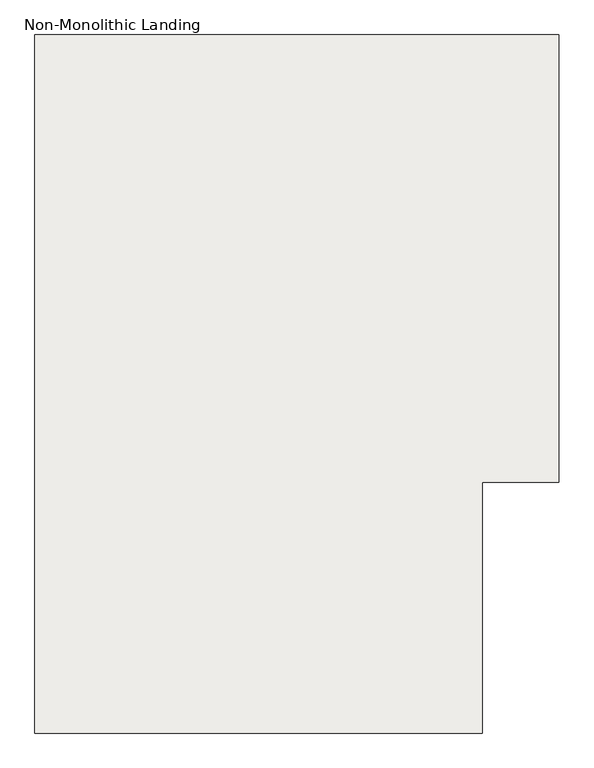
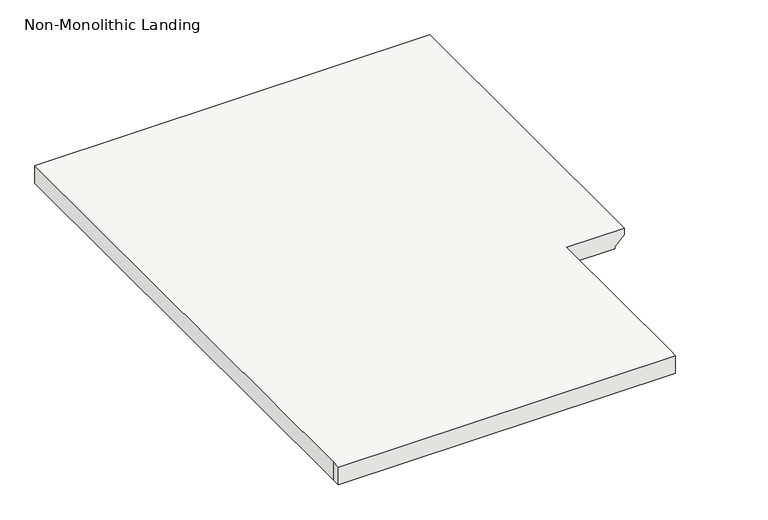
"""IFC4 building model written with IfcOpenShell, lengths in millimetres: slab geometry, Non-Monolithic Landing."""

from ifc_helpers import new_model, si_unit, origin, place, context, project, spatial, faceted_brep, source, transform, mapped, element, save


def non_monolithic_landing_30da2899(model_context):
    return source(origin(), model_context, "Body", "Brep", [
        faceted_brep([(-10197.3156858, 1045.1115003, 4180.4166667), (-10197.3156858, 1045.1115003, 4199.4666667), (-10197.3156858, 130.7115003, 4199.4666667), (-10197.3156858, 130.7115003, 4180.4166667), (-10222.7156858, 1045.1115003, 4155.0166667), (-10222.7156858, 130.7115003, 4155.0166667), (-11268.1522729, 1045.1115003, 4199.4666667), (-11268.1522729, -356.3993654, 4199.4666667), (-11268.1522729, -381.7993654, 4199.4666667), (-10353.7522729, -381.7993654, 4199.4666667), (-10353.7522729, -356.3993654, 4199.4666667), (-10353.7522729, 130.7115003, 4199.4666667), (-10222.7156858, 1045.1115003, 4148.6666667), (-10222.7156858, 130.7115003, 4148.6666667), (-10353.7522729, 130.7115003, 4148.6666667), (-10353.7522729, -356.3993654, 4148.6666667), (-10353.7522729, -381.7993654, 4148.6666667), (-11268.1522729, -381.7993654, 4148.6666667), (-11268.1522729, -356.3993654, 4148.6666667), (-11268.1522729, 1045.1115003, 4148.6666667)], [[[0, 1, 2, 3]], [[4, 0, 3, 5]], [[6, 7, 8, 9, 10, 11, 2, 1]], [[12, 13, 14, 15, 16, 17, 18, 19]], [[13, 12, 4, 5]], [[6, 1, 0, 4, 12, 19]], [[7, 6, 19, 18]], [[8, 7, 18, 17]], [[9, 8, 17, 16]], [[10, 9, 16, 15]], [[11, 10, 15, 14]], [[2, 11, 14, 13, 5, 3]]]),
    ])


if __name__ == "__main__":
    model = new_model("IFC4")
    model_context = context("Model", 3, world=origin())
    ifc_project = project(units=[si_unit("LENGTHUNIT", "METRE", prefix="MILLI")], contexts=[model_context])
    site = spatial("IfcSite", under=ifc_project)
    building = spatial("IfcBuilding", under=site)
    placement = place(None, origin())
    non_monolithic_landing_shape = non_monolithic_landing_30da2899(model_context)
    element("IfcSlab", 1, ObjectType="Non-Monolithic Landing", at=placement, inside=building, context=model_context, shape_type="MappedRepresentation", body=[
        mapped(non_monolithic_landing_shape, transform((0.0, 0.0, 0.0), x_axis=(1.0, 0.0, 0.0), y_axis=(0.0, 1.0, 0.0), z_axis=(0.0, 0.0, 1.0))),
    ])
    save(model, "model.ifc")
